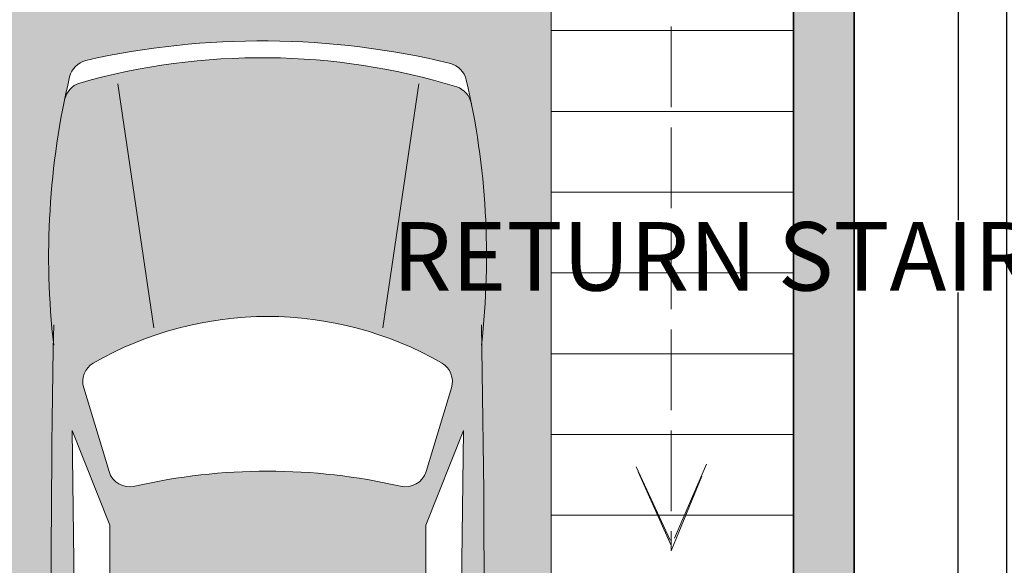
# Model space of a CAD drawing. Units: inches. Extents: x 1077 to 2505, y 1892 to 2728.
# Tile 8 of 26: x 1433 to 1579, y 2176 to 2257. Entities that reach past the tile are written whole.
import ezdxf

# ---------------------------------------------------------------- set-up
doc = ezdxf.new("R2010")
doc.units = ezdxf.units.IN
doc.linetypes.add('ACAD_ISO02W100', pattern=[15, 12, -3])
doc.layers.get('Defpoints').update_dxf_attribs({"color": 220, "linetype": 'ACAD_ISO02W100'})
for name, color, linetype, lineweight in [('A-ANNO-DIMS', 2, 'Continuous', 18), ('A-ANNO-STRS', 220, 'ACAD_ISO02W100', 13), ('A-FLOR-FIXT', 8, 'Continuous', 13), ('A-FLOR-STRS', 7, 'Continuous', 18), ('A-FURNITURE', 251, 'Continuous', 5), ('A-SITE-VEHI', 8, 'Continuous', 13), ('A-WALL-PATT', 7, 'Continuous', 9), ('A_TEXT_SMALL', 18, 'Continuous', 13), ('WALL', 7, 'Continuous', 35)]:
    doc.layers.add(name, color=color, linetype=linetype, lineweight=lineweight)
doc.layers.add('A-FLOR-PATT', color=254, linetype='Continuous', lineweight=9, true_color=0xd7ebd2)
doc.styles.get("Standard").update_dxf_attribs({"font": 'arial.ttf'})
doc.dimstyles.get("Standard").update_dxf_attribs({"dimtxt": 10.18, "dimasz": 0.18, "dimexe": 0.18, "dimexo": 0.0625, "dimgap": 0.09, "dimtad": 0, "dimtih": 1, "dimtoh": 1, "dimdec": 0, "dimzin": 0, "dimdsep": 46, "dimlunit": 3, "dimtxsty": 'Standard', "dimcen": 0.09, "dimadec": 0, "dimazin": 0, "dimtfac": 1, "dimtdec": 0, "dimtofl": 0, "dimtmove": 0, "dimatfit": 3, "dimfxl": 1, "dimtolj": 1, "dimtzin": 0, "dimarcsym": 0})

# ---------------------------------------------------------------- blocks, each defined once
blk = doc.blocks.new('CAR')
at = {"layer": 'A-FURNITURE'}
for p, q in [((2677.91, 1665.57), (2683.24, 1629.33)), ((2722.63, 1665.57), (2717.3, 1629.33)), ((2672.85, 1620.44), (2676.61, 1608)), ((2727.48, 1620.44), (2723.73, 1608)), ((2671.15, 1614.07), (2676.73, 1600.01)), ((2671.63, 1575.61), (2671.15, 1614.07)), ((2729.25, 1614.07), (2723.67, 1600.01)), ((2728.77, 1575.61), (2729.25, 1614.07)), ((2676.73, 1600.01), (2676.73, 1578.97)), ((2723.67, 1600.01), (2723.67, 1578.97)), ((2676.73, 1578.97), (2671.63, 1575.61)), ((2723.67, 1578.97), (2728.77, 1575.61)), ((2676.73, 1576.71), (2671.66, 1573.38)), ((2676.73, 1576.71), (2676.73, 1555.46)), ((2723.67, 1576.71), (2723.67, 1555.46)), ((2723.67, 1576.71), (2728.74, 1573.38)), ((2671.9, 1540.91), (2671.66, 1573.38)), ((2728.49, 1540.91), (2728.74, 1573.38)), ((2676.73, 1555.46), (2671.9, 1540.91)), ((2723.67, 1555.46), (2728.49, 1540.91)), ((2678.77, 1552.01), (2672.52, 1524.85)), ((2721.71, 1552.02), (2727.96, 1524.85)), ((2675.22, 1526.01), (2679.74, 1548.74)), ((2725.17, 1526.01), (2720.66, 1548.74)), ((2672.52, 1524.85), (2672.52, 1517.39)), ((2727.96, 1524.85), (2727.96, 1517.39))]:
    blk.add_line(p, q, dxfattribs=at)
for centre, radius, start, end in [((2699.3, 1552.83), 119.14, 76.3976, 102.667), ((2699.3, 1570.19), 99.28, 73.0347, 105.8141), ((2674, 1665.84), 3.34, 104.3452, 166.6607), ((2726.43, 1665.41), 3.34, 13.1156, 74.5941), ((2783.1, 1639.97), 115.47, 166.6607, 186.5655), ((2673.27, 1662.52), 3.34, 107.8179, 168.3942), ((2727.17, 1661.99), 3.34, 11.3249, 70.8826), ((2617.23, 1639.97), 115.47, 353.4345, 13.1156), ((2700.17, 1579.09), 51.94, 60.0774, 119.9226), ((4741.11, 1589.62), 2073.11, 178.89024, 182.01225), ((659.22, 1589.62), 2073.11, 357.98775, 1.10976), ((2675.91, 1621.37), 3.2, 121.1455, 196.7984), ((2724.42, 1621.37), 3.2, 343.2016, 58.8545), ((2679.67, 1608.92), 3.2, 196.7984, 283.6631), ((2700.17, 1519.83), 88.22, 77.0683, 102.9317), ((2720.66, 1608.92), 3.2, 256.3369, 343.2016), ((2700.16, 1829.45), 278.26, 265.5919, 274.4407), ((2700.17, 1827.63), 279.65, 265.7971, 274.2029), ((2700.17, 1663.47), 139.72, 259.6897, 280.3103), ((2674.03, 1521.04), 4.9, 184.3987, 237.5288), ((2726.3, 1521.04), 4.9, 302.4712, 355.6013), ((2672.62, 1516.95), 3.34, 182.1119, 263.4899), ((2700.17, 1791.26), 275.86, 264.0142, 275.9858), ((2727.71, 1516.95), 3.34, 276.5101, 357.8881), ((2700.17, 1790.18), 277.96, 264.2342, 275.7658)]:
    blk.add_arc(centre, radius, start, end, dxfattribs=at)
blk = doc.blocks.new('reh-flat-2')
at = {"layer": 'A_TEXT_SMALL'}
for p, q in [((486053827.2, -394630231.2), (486054182.4, -394629799.8)), ((486054182.4, -394629799.8), (486054596.6, -394630140.9)), ((486053979.5, -394630126.3), (486054157.1, -394629910.6)), ((486054228.6, -394629903.6), (486054483.5, -394630113.5)), ((486054596.6, -394630140.9), (486054241.4, -394630572.3)), ((486054241.3, -394630407.7), (486053986.4, -394630197.8)), ((486054490.4, -394630185), (486054312.8, -394630400.7)), ((486054241.4, -394630572.3), (486053827.2, -394630231.2))]:
    blk.add_line(p, q, dxfattribs=at)
for centre, radius in [((486054234.9, -394630155.7), 38.1), ((486054004.1, -394630296.2), 20.1), ((486054072.7, -394630352.7), 20.1), ((486054141.4, -394630409.3), 20.1)]:
    blk.add_circle(centre, radius, dxfattribs=at)
for centre, start, end in [((486054196.3, -394629942.9), 50.5305, 140.5305), ((486054018.7, -394630158.5), 140.5305, 230.5305), ((486054451.2, -394630152.8), 320.5305, 50.5305), ((486054273.6, -394630368.4), 230.5305, 320.5305)]:
    blk.add_arc(centre, 50.8, start, end, dxfattribs=at)
blk = doc.blocks.new('*D14')
at = {"layer": 'A-ANNO-DIMS', "color": 0, "lineweight": -2, "transparency": 16777216}
for p, q in [((1555.59, 2651.66), (1579.43, 2651.66)), ((1579.25, 2651.48), (1579.25, 2375.3)), ((1579.25, 2088.54), (1579.25, 2364.72)), ((1555.59, 2088.36), (1579.43, 2088.36))]:
    blk.add_line(p, q, dxfattribs=at)
at = {"layer": 'A-ANNO-DIMS', "color": 0, "transparency": 16777216}
for points in [[(1579.22, 2651.48), (1579.28, 2651.48), (1579.25, 2651.66)], [(1579.22, 2088.54), (1579.28, 2088.54), (1579.25, 2088.36)]]:
    blk.add_solid(points, dxfattribs=at)
at = {"layer": 'Defpoints', "color": 0, "transparency": 16777216}
for p in [(1555.53, 2651.66), (1555.53, 2088.36), (1579.25, 2088.36)]:
    blk.add_point(p, dxfattribs=at)
at = {"layer": 'A-ANNO-DIMS', "color": 0, "transparency": 16777216, "insert": (1579.25, 2370.01), "char_height": 10.18, "attachment_point": 5}
blk.add_mtext('\\A1;46\'-11"', dxfattribs=at)
blk = doc.blocks.new('STAIR-PLAN-RETURN')
for p, q in [((36, 163.08), (36, 0)), ((36, 115.08), (72, 115.08)), ((36, 103.08), (72, 103.08)), ((36, 91.08), (72, 91.08)), ((36, 79.08), (72, 79.08)), ((36, 67.08), (72, 67.08)), ((36, 55.08), (72, 55.08)), ((36, 43.08), (72, 43.08))]:
    blk.add_line(p, q)
blk = doc.blocks.new('STAIR-DIRECTION')
for p, q in [((0, 107.9), (70.51, 107.9)), ((70.51, 107.9), (70.51, 0)), ((70.51, 0.8), (65.28, 12.48)), ((65.28, 12.48), (70.51, 1.21)), ((70.51, 0), (75.75, 12.88)), ((75.75, 12.88), (70.51, 0.8))]:
    blk.add_line(p, q)
blk = doc.blocks.new('*D44')
at = {"layer": 'A-ANNO-DIMS', "color": 0, "lineweight": -2, "transparency": 16777216}
for p, q in [((1547.59, 2303.16), (1572.17, 2303.16)), ((1571.99, 2302.98), (1571.99, 2226.98)), ((1571.99, 2140.26), (1571.99, 2216.26)), ((1547.59, 2140.08), (1572.17, 2140.08))]:
    blk.add_line(p, q, dxfattribs=at)
at = {"layer": 'A-ANNO-DIMS', "color": 0, "transparency": 16777216}
for points in [[(1571.96, 2302.98), (1572.02, 2302.98), (1571.99, 2303.16)], [(1571.96, 2140.26), (1572.02, 2140.26), (1571.99, 2140.08)]]:
    blk.add_solid(points, dxfattribs=at)
at = {"layer": 'Defpoints', "color": 0, "transparency": 16777216}
for p in [(1547.53, 2303.16), (1571.99, 2303.16), (1547.53, 2140.08)]:
    blk.add_point(p, dxfattribs=at)
at = {"layer": 'A-ANNO-DIMS', "color": 0, "transparency": 16777216, "insert": (1571.99, 2221.62), "char_height": 10.18, "attachment_point": 5}
blk.add_mtext('\\A1;RETURN STAIR 13\'-7" TYP.', dxfattribs=at)

msp = doc.modelspace()

# ---------------------------------------------------------------- hatches: boundary and pattern name
at = {"layer": 'A-FLOR-PATT', "transparency": 33554559}
h = msp.add_hatch(color=256, dxfattribs=at)
h.dxf.hatch_style = 1
h.paths.add_polyline_path([(1395.53, 2577.16), (1374.83, 2577.16), (1350.83, 2577.19), (1350.83, 2577.16), (1329.53, 2577.16), (1329.53, 2480.16), (1329.53, 2469.16), (1325.53, 2469.16), (1325.53, 2515.13), (1307.53, 2515.13), (1307.53, 2577.16), (1269.31, 2577.16), (1221.31, 2577.15), (1221.31, 2577.16), (1187.53, 2577.16), (1187.53, 2433.16), (1289.53, 2433.16), (1289.53, 2429.16), (1263.53, 2429.16), (1187.53, 2429.16), (1187.53, 2395.02), (1187.53, 2395.02), (1187.53, 2371.02), (1187.53, 2371.02), (1187.53, 2307.16), (1259.53, 2307.16), (1259.53, 2399.16), (1263.53, 2399.16), (1263.53, 2307.16), (1289.53, 2307.16), (1289.53, 2306.23), (1325.53, 2306.23), (1325.53, 2307.16), (1329.53, 2307.16), (1329.53, 2306.23), (1365.53, 2306.23), (1365.53, 2307.16), (1432.53, 2307.16), (1432.53, 2088.16), (1547.53, 2088.16), (1547.53, 2140.08), (1511.53, 2140.08), (1511.53, 2267.16), (1475.53, 2267.16), (1475.53, 2303.16), (1468.53, 2303.16), (1468.53, 2307.16), (1547.53, 2307.16), (1547.53, 2348.22), (1547.53, 2396.22), (1547.53, 2429.16), (1435.53, 2429.16), (1435.53, 2433.16), (1476.35, 2433.16), (1476.35, 2451.18), (1547.53, 2451.18), (1547.53, 2577.16), (1499.53, 2577.16), (1499.53, 2586.16), (1547.53, 2586.16), (1547.53, 2642.16), (1518.18, 2642.16), (1518.18, 2642.05), (1494.15, 2642.05), (1494.15, 2642.16), (1469.53, 2642.16), (1469.53, 2577.16), (1399.53, 2577.16), (1399.53, 2429.16), (1325.53, 2429.16), (1325.53, 2433.16), (1329.53, 2433.16), (1395.53, 2433.16), (1395.53, 2480.16), (1359.53, 2480.16), (1359.53, 2484.16), (1395.53, 2484.16)])
h.paths.add_polyline_path([(1357.65, 2482.07), (1355.65, 2482.07), (1355.65, 2481.07, 0.414214), (1356.65, 2480.07), (1344.65, 2480.07), (1344.65, 2477.06), (1343.27, 2477.06), (1343.27, 2480.07), (1330.65, 2480.07, -0.414214), (1329.65, 2481.07), (1329.65, 2484.07), (1331.65, 2484.07), (1331.65, 2510.07, -0.446908)], flags=16)
h.paths.add_polyline_path([(1305.09, 2559.18), (1288.89, 2559.18), (1288.89, 2575.38), (1305.09, 2575.38)], flags=16)
h.paths.add_polyline_path([(1304.19, 2560.08), (1289.79, 2560.08), (1289.79, 2574.48), (1304.19, 2574.48)], flags=0)
h.paths.add_polyline_path([(1287.99, 2500.68, -0.414214), (1287.09, 2499.78), (1265.14, 2499.78), (1224.09, 2499.78, -0.414214), (1223.19, 2500.68), (1223.19, 2557.16), (1223.19, 2571.74), (1223.19, 2575.38), (1287.99, 2575.38), (1287.99, 2571.74), (1287.09, 2571.74, -0.414214), (1287.99, 2570.84)], flags=16)
h.paths.add_polyline_path([(1292.98, 2569.05, -1), (1300.92, 2569.05, -1)], flags=0)
h.paths.add_polyline_path([(1293.32, 2569.05, -1), (1300.58, 2569.05, -1)], flags=0)
h.paths.add_polyline_path([(1322.8, 2462.21), (1322.8, 2431.71), (1323.05, 2430.71), (1323.05, 2431.71), (1321.8, 2431.71), (1321.8, 2462.19, 0.404641), (1292.3, 2431.71), (1292.05, 2430.71, -0.414214), (1291.55, 2430.21), (1291.05, 2430.21), (1291.05, 2429.71, -0.414214), (1290.55, 2429.21), (1289.55, 2429.21), (1289.55, 2434.21), (1290.55, 2434.21, -0.414214), (1291.05, 2433.71), (1291.05, 2433.21), (1291.55, 2433.21, -0.414214), (1292.05, 2432.71), (1292.3, 2431.71, -0.414214)], flags=16)
h.paths.add_polyline_path([(1287.82, 2548.28, 0.292232), (1279.17, 2536.8, 0.052719), (1223.93, 2548.28), (1223.28, 2548.28), (1223.28, 2557.16), (1223.93, 2557.16), (1245.42, 2557.16, -0.117785), (1245.77, 2557.93, -0.059418), (1254.87, 2567.02, -0.379859), (1257.28, 2566.88, -0.02509), (1261.41, 2563.32, -0.025935), (1265.65, 2567.02, -0.379859), (1268.06, 2566.88, -0.061767), (1277.52, 2557.43, -0.069393), (1277.82, 2557.16), (1287.82, 2557.16)], flags=0)
h.paths.add_polyline_path([(1263.47, 2548.28), (1260.56, 2548.28, -0.015371), (1258.01, 2546.13, -0.429576), (1255.37, 2546.06, -0.016036), (1252.69, 2548.28), (1223.28, 2548.28), (1223.28, 2554.42), (1246.78, 2554.42, 0.055344), (1255.37, 2546.06, 0.331768), (1257.52, 2545.74, 0.027343), (1262, 2549.64, 0.00919)], flags=0)
h.paths.add_polyline_path([(1295.56, 2568.34), (1296.87, 2569.09), (1296.87, 2570.6, 0.399698), (1295.39, 2569.05, 0.119004)], flags=0)
h.paths.add_polyline_path([(1295.21, 2569.05, -1), (1298.68, 2569.05, -1)], flags=0)
h.paths.add_polyline_path([(1296.95, 2568.96), (1297.03, 2569), (1297.03, 2569.09), (1296.99, 2569.11), (1296.91, 2568.98)], flags=0)
h.paths.add_polyline_path([(1402.28, 2462.19, -0.414214), (1432.78, 2431.69), (1433.03, 2432.69), (1432.78, 2431.69, 0.404641), (1403.28, 2462.17), (1403.28, 2431.69), (1402.03, 2431.69), (1402.03, 2430.69, -0.414214), (1401.53, 2430.19), (1401.03, 2430.19), (1401.03, 2429.69, -0.414214), (1400.53, 2429.19), (1399.53, 2429.19), (1399.53, 2434.19), (1400.53, 2434.19, -0.414214), (1401.03, 2433.69), (1401.03, 2433.19), (1401.53, 2433.19, -0.414214), (1402.03, 2432.69)], flags=16)
h.paths.add_polyline_path([(1470.16, 2535.21, -0.414214), (1471.06, 2536.11), (1527.54, 2536.11), (1542.12, 2536.11), (1545.76, 2536.11), (1545.76, 2471.31), (1542.12, 2471.31), (1542.12, 2472.21, -0.414214), (1541.22, 2471.31), (1471.06, 2471.31, -0.414214), (1470.16, 2472.21), (1470.16, 2494.16)], flags=16)
h.paths.add_polyline_path([(1483.07, 2536.11, 0.253465), (1480.11, 2526.15, 0.2538), (1470.15, 2523.19)], flags=16)
h.paths.add_polyline_path([(1223.19, 2512.69, 0.253465), (1233.14, 2509.74, 0.2538), (1236.1, 2499.77)], flags=16)
h.paths.add_polyline_path([(1469.77, 2578.72), (1469.77, 2581.72), (1471.77, 2581.72), (1471.77, 2607.72, -0.01951), (1473.77, 2607.68), (1473.77, 2579.72), (1473.77, 2578.72, -0.414214), (1472.77, 2577.72), (1470.77, 2577.72, -0.414214)], flags=16)
h.paths.add_polyline_path([(1382.46, 2398.13), (1395.04, 2398.13), (1395.04, 2399.74), (1382.46, 2399.74)], flags=16)
h.paths.add_polyline_path([(1379.94, 2397.18), (1379.94, 2389.82), (1380.5, 2389.82), (1380.5, 2396.05, -0.41429), (1381.06, 2396.61), (1396.47, 2396.61, -0.414213), (1397.03, 2396.05), (1397.03, 2389.82), (1397.59, 2389.82), (1397.59, 2397.18)], flags=16)
h.paths.add_polyline_path([(1263.37, 2428.14), (1263.37, 2426.14, -0.414214), (1262.37, 2425.14), (1261.37, 2425.14), (1233.41, 2425.14, 0.400854), (1259.37, 2401.04), (1259.37, 2401.14), (1261.37, 2401.14, -0.446908), (1233.37, 2427.14), (1259.37, 2427.14), (1259.37, 2429.14), (1262.37, 2429.14, -0.414214)], flags=16)
h.paths.add_polyline_path([(1404.79, 2398.13), (1417.37, 2398.13), (1417.37, 2399.74), (1404.79, 2399.74)], flags=16)
h.paths.add_polyline_path([(1402.27, 2397.18), (1404.79, 2398.13), (1417.37, 2398.13), (1419.92, 2397.18)], flags=16)
h.paths.add_polyline_path([(1432.26, 2383.16), (1432.26, 2370.59), (1433.87, 2370.59), (1433.87, 2383.16)], flags=16)
h.paths.add_polyline_path([(1431.3, 2385.69), (1423.84, 2385.69), (1423.84, 2385.13), (1430.18, 2385.13, -0.41429), (1430.74, 2384.57), (1430.74, 2369.16, -0.414237), (1430.18, 2368.6), (1423.84, 2368.6), (1423.84, 2368.03), (1431.3, 2368.03)], flags=16)
h.paths.add_polyline_path([(1417.37, 2351.16), (1417.37, 2349.54), (1418.9, 2349.54, 0.414236), (1419.92, 2350.56), (1419.92, 2352.11)], flags=16)
h.paths.add_polyline_path([(1395.04, 2351.16), (1395.04, 2349.54), (1396.58, 2349.54, 0.414235), (1397.59, 2350.56), (1397.59, 2352.11)], flags=16)
h.paths.add_polyline_path([(1366.7, 2370.05), (1365.09, 2370.05), (1365.09, 2368.52, 0.414235), (1366.11, 2367.5), (1367.66, 2367.5)], flags=16)
h.paths.add_polyline_path([(1419.36, 2359.47), (1419.36, 2353.24, -0.41419), (1418.8, 2352.68), (1403.39, 2352.68, -0.414137), (1402.83, 2353.24), (1402.83, 2359.47), (1397.03, 2359.47), (1397.03, 2353.24, -0.414189), (1396.47, 2352.68), (1381.06, 2352.68, -0.414137), (1380.5, 2353.24), (1380.5, 2359.47)], flags=16)
h.paths.add_polyline_path([(1222.29, 2559.18), (1206.09, 2559.18), (1206.09, 2575.38), (1222.29, 2575.38)], flags=16)
h.paths.add_polyline_path([(1221.39, 2560.08), (1206.99, 2560.08), (1206.99, 2574.48), (1221.39, 2574.48)], flags=0)
h.paths.add_polyline_path([(1482, 2577.72), (1482, 2580.73), (1483.38, 2580.73), (1483.38, 2577.72), (1484.77, 2577.72), (1484.77, 2574.72), (1483.38, 2574.72), (1483.38, 2577.72)], flags=16)
h.paths.add_polyline_path([(1266.37, 2415.53), (1266.37, 2414.14), (1263.37, 2414.14), (1263.37, 2415.53), (1260.36, 2415.53), (1260.36, 2416.91), (1263.37, 2416.91), (1263.37, 2415.53)], flags=16)
h.paths.add_polyline_path([(1210.26, 2569.05, -1), (1218.19, 2569.05, -1)], flags=0)
h.paths.add_polyline_path([(1210.6, 2569.05, -1), (1217.85, 2569.05, -1)], flags=0)
h.paths.add_polyline_path([(1212.84, 2568.34), (1214.15, 2569.09), (1214.15, 2570.6, 0.399698), (1212.67, 2569.05, 0.119004)], flags=0)
h.paths.add_polyline_path([(1212.49, 2569.05, -1), (1215.96, 2569.05, -1)], flags=0)
h.paths.add_polyline_path([(1214.23, 2568.96), (1214.3, 2568.91), (1214.3, 2569)], flags=0)
h.paths.add_polyline_path([(1507.18, 2480.12, 0.052719), (1518.66, 2535.36), (1518.66, 2536.01), (1527.54, 2536.01), (1527.54, 2535.36), (1527.54, 2513.88, -0.117785), (1528.31, 2513.53, -0.059418), (1537.4, 2504.43, -0.379859), (1537.26, 2502.01, -0.02509), (1533.7, 2497.89, -0.025935), (1537.4, 2493.64, -0.379859), (1537.26, 2491.23, -0.061767), (1527.8, 2481.77, -0.069393), (1527.54, 2481.47), (1527.54, 2471.47), (1518.66, 2471.47, 0.292232)], flags=0)
h.paths.add_polyline_path([(1516.43, 2503.92, -0.016036), (1518.66, 2506.6), (1518.66, 2536.01), (1524.8, 2536.01), (1524.8, 2512.51, 0.055344), (1516.43, 2503.92, 0.331768), (1516.12, 2501.77, 0.027343), (1520.01, 2497.29, 0.00919), (1518.66, 2495.82), (1518.66, 2498.73, -0.015371), (1516.5, 2501.28, -0.429576)], flags=0)
h.paths.add_polyline_path([(1499.63, 2625.5, -0.171636), (1502.82, 2631.01), (1502.82, 2633.37), (1498.68, 2633.37, -0.414214), (1497.7, 2634.36), (1497.7, 2640.66, -0.414214), (1498.68, 2641.64), (1514.82, 2641.64, -0.414214), (1515.81, 2640.66), (1515.81, 2634.36, -0.414214), (1514.82, 2633.37), (1510.69, 2633.37), (1510.69, 2631.01, -0.171636), (1513.88, 2625.5, -0.258205), (1509.31, 2614.47), (1504.19, 2614.47, -0.258205)], flags=16)
h.paths.add_polyline_path([(1501.2, 2625.5, -0.171636), (1504.39, 2631.01), (1509.12, 2631.01, -0.171636), (1512.3, 2625.5, -0.210384), (1509.35, 2616.02), (1504.16, 2616.02, -0.210384)], flags=0)
h.paths.add_polyline_path([(1529.56, 2537.01), (1529.56, 2553.21), (1545.76, 2553.21), (1545.76, 2537.01)], flags=16)
h.paths.add_polyline_path([(1530.46, 2537.91), (1530.46, 2552.31), (1544.86, 2552.31), (1544.86, 2537.91)], flags=0)
h.paths.add_polyline_path([(1535.45, 2545.07, -1), (1543.39, 2545.07, -1)], flags=0)
h.paths.add_polyline_path([(1535.8, 2545.07, -1), (1543.05, 2545.07, -1)], flags=0)
h.paths.add_polyline_path([(1529.56, 2470.41), (1545.76, 2470.41), (1545.76, 2454.21), (1529.56, 2454.21)], flags=16)
h.paths.add_polyline_path([(1541.16, 2544.99), (1540.98, 2544.99, -0.544606), (1538.71, 2543.68), (1538.62, 2543.53, 0.547962)], flags=0)
h.paths.add_polyline_path([(1530.46, 2469.51), (1544.86, 2469.51), (1544.86, 2455.11), (1530.46, 2455.11)], flags=0)
h.paths.add_polyline_path([(1539.47, 2545.14), (1539.42, 2545.22), (1539.38, 2545.14)], flags=0)
h.paths.add_polyline_path([(1543.39, 2462.34, -1), (1535.45, 2462.34, -1)], flags=0)
h.paths.add_polyline_path([(1543.05, 2462.34, -1), (1535.8, 2462.34, -1)], flags=0)
h.paths.add_polyline_path([(1541.16, 2462.27), (1540.98, 2462.27, -0.544606), (1538.71, 2460.96), (1538.62, 2460.8, 0.547962)], flags=0)
h.paths.add_polyline_path([(1539.47, 2462.42), (1539.42, 2462.5), (1539.38, 2462.42)], flags=0)
h.paths.add_polyline_path([(1435.32, 2335.25, -0.414214), (1465.82, 2304.75), (1466.07, 2305.75), (1465.82, 2304.75, 0.404641), (1436.32, 2335.23), (1436.32, 2304.75), (1435.07, 2304.75), (1435.07, 2303.75, -0.414214), (1434.57, 2303.25), (1434.07, 2303.25), (1434.07, 2302.75, -0.414214), (1433.57, 2302.25), (1432.57, 2302.25), (1432.57, 2307.25), (1433.57, 2307.25, -0.414214), (1434.07, 2306.75), (1434.07, 2306.25), (1434.57, 2306.25, -0.414214), (1435.07, 2305.75)], flags=16)
h.paths.add_polyline_path([(1532.13, 2635.71), (1535.43, 2635.71), (1535.43, 2635.89), (1532.13, 2635.89)], flags=16)
edge = h.paths.add_edge_path(flags=16)
edge.add_arc((1535.98, 2632.67), 0.183, 270, 360)
edge.add_line((1536.17, 2632.67), (1536.17, 2639.82))
edge.add_line((1536.17, 2639.82), (1538.29, 2639.82))
edge.add_line((1538.29, 2639.82), (1538.29, 2641.82))
edge.add_line((1538.29, 2641.82), (1533.25, 2641.82))
edge.add_line((1533.25, 2641.82), (1533.25, 2639.82))
edge.add_line((1533.25, 2639.82), (1534.87, 2639.82))
edge.add_line((1534.87, 2639.82), (1534.87, 2639))
edge.add_line((1534.87, 2639), (1533.7, 2639))
edge.add_line((1533.7, 2639), (1533.7, 2639.82))
edge.add_line((1533.7, 2639.82), (1533.25, 2639.82))
edge.add_line((1533.25, 2639.82), (1533.25, 2641.82))
edge.add_line((1533.25, 2641.82), (1538.29, 2641.82))
edge.add_line((1538.29, 2641.82), (1538.29, 2641.34))
edge.add_line((1538.29, 2641.34), (1540.64, 2641.58))
edge.add_line((1540.64, 2641.58), (1540.64, 2641.82))
edge.add_line((1540.64, 2641.82), (1541.5, 2641.82))
edge.add_line((1541.5, 2641.82), (1541.5, 2641.25))
edge.add_line((1541.5, 2641.25), (1541.31, 2639.79))
edge.add_ellipse((1541.09, 2638.95), major_axis=(-1.08, 0), ratio=0.790849, start_angle=180, end_angle=255.2976, ccw=False)
edge.add_line((1542.17, 2638.95), (1542.17, 2638.38))
edge.add_ellipse((1541.09, 2638.38), major_axis=(-1.08, 0), ratio=0.790849, start_angle=0, end_angle=180, ccw=False)
edge.add_line((1540, 2638.38), (1540.01, 2638.87))
edge.add_ellipse((1541.09, 2638.95), major_axis=(-1.08, 0), ratio=0.790849, start_angle=284.7024, end_angle=364.0401, ccw=False)
edge.add_line((1540.78, 2639.75), (1540.78, 2641.25))
edge.add_line((1540.78, 2641.25), (1540.64, 2641.25))
edge.add_line((1540.64, 2641.25), (1538.29, 2641.01))
edge.add_line((1538.29, 2641.01), (1538.29, 2639.82))
edge.add_line((1538.29, 2639.82), (1536.17, 2639.82))
edge.add_line((1536.17, 2639.82), (1536.17, 2632.48))
edge.add_line((1536.17, 2632.48), (1535.98, 2632.48))
h.paths.add_polyline_path([(1496.32, 2250.34, -0.292371), (1498.9, 2247.83, -0.085148), (1501.21, 2208.85, -0.01331), (1500.27, 2098.5, -0.379287), (1497.22, 2095.28, -0.0502), (1441.54, 2095.28, -0.379287), (1438.5, 2098.5, -0.01331), (1437.56, 2208.85, -0.086132), (1439.96, 2248.26, -0.295116), (1442.59, 2250.78, -0.114238)], flags=16)
h.paths.add_polyline_path([(1495.16, 2205.84, -0.355389), (1496.7, 2202.1), (1492.94, 2189.65, -0.398275), (1489.12, 2187.47, 0.113332), (1449.64, 2187.47, -0.398275), (1445.82, 2189.65), (1442.06, 2202.1, -0.355394), (1443.6, 2205.84, -0.265725)], flags=0)
h.paths.add_polyline_path([(1440.37, 2195.72), (1445.94, 2181.67), (1445.94, 2160.63), (1440.84, 2157.26)], flags=0)
h.paths.add_polyline_path([(1498.46, 2195.72), (1497.99, 2157.26), (1492.88, 2160.63), (1492.88, 2181.67)], flags=0)
h.paths.add_polyline_path([(1445.94, 2158.37), (1445.94, 2137.12), (1441.12, 2122.56), (1440.87, 2155.03)], flags=0)
h.paths.add_polyline_path([(1492.88, 2158.37), (1497.96, 2155.03), (1497.71, 2122.56), (1492.88, 2137.12)], flags=0)
h.paths.add_polyline_path([(1489.88, 2130.4), (1494.39, 2107.67, -0.090102), (1444.44, 2107.65), (1448.95, 2130.39, 0.036636)], flags=0)
h.paths.add_polyline_path([(1447.54, 2159.34), (1497.44, 2159.34), (1497.44, 2177.89), (1447.54, 2177.89)], flags=8)
h.paths.add_polyline_path([(1196.44, 2354.84), (1246.65, 2354.84), (1246.65, 2388.43), (1196.44, 2388.43)], flags=24)
h.paths.add_polyline_path([(1296.09, 2360.25), (1353.81, 2360.25), (1353.81, 2393.84), (1296.09, 2393.84)], flags=24)
h.paths.add_polyline_path([(1400.72, 2471.85), (1470.63, 2471.85), (1470.63, 2505.44), (1400.72, 2505.44)], flags=24)
h.paths.add_polyline_path([(1324.78, 2448.48), (1394.95, 2448.48), (1394.95, 2467.02), (1324.78, 2467.02)], flags=24)
h.paths.add_polyline_path([(1335.08, 2531.43), (1389.67, 2531.43), (1389.67, 2565.02), (1335.08, 2565.02)], flags=24)
h.paths.add_polyline_path([(1225.76, 2460), (1295.67, 2460), (1295.67, 2493.58), (1225.76, 2493.58)], flags=24)
h = msp.add_hatch(color=256, dxfattribs=at)
h.dxf.hatch_style = 1
h.paths.add_polyline_path([(1547.53, 2348.22), (1547.53, 2396.22), (1547.53, 2425.11), (1547.53, 2425.11), (1547.53, 2429.16), (1435.53, 2429.16), (1434.03, 2429.21), (1434.03, 2430.19), (1433.03, 2430.19), (1432.78, 2431.69, 0.404641), (1403.28, 2462.17), (1403.28, 2431.69), (1402.03, 2431.69), (1402.03, 2430.19), (1401.03, 2430.19), (1401.03, 2429.19), (1399.53, 2429.19), (1399.53, 2429.19), (1399.53, 2429.16), (1334.67, 2429.16), (1334.67, 2423.95), (1325.67, 2423.95), (1325.67, 2429.16), (1325.53, 2429.16), (1324.05, 2429.24), (1324.05, 2430.21), (1323.05, 2430.21), (1323.05, 2431.71), (1321.8, 2431.71), (1321.8, 2462.19, 0.416544), (1292.05, 2430.73, -0.423614), (1291.55, 2430.21), (1291.05, 2430.21), (1291.05, 2429.21), (1289.55, 2429.21), (1289.53, 2429.21), (1289.53, 2429.16), (1263.37, 2429.16), (1263.37, 2415.53), (1266.37, 2415.53), (1266.37, 2414.14), (1263.37, 2414.14), (1263.37, 2399.16), (1263.53, 2399.16), (1263.53, 2307.16), (1289.53, 2307.16), (1289.53, 2306.23), (1323.26, 2306.23), (1323.26, 2307.21), (1332.26, 2307.21), (1365.53, 2306.23), (1365.53, 2307.16), (1432.53, 2307.16), (1432.57, 2307.16), (1432.57, 2307.25), (1434.07, 2307.25), (1434.07, 2306.25), (1435.32, 2306.25), (1435.32, 2335.25, -0.407346), (1466.07, 2305.73, -0.423614), (1466.57, 2306.25), (1467.07, 2306.25), (1467.07, 2307.25), (1468.57, 2307.25), (1547.53, 2307.16), (1547.53, 2307.2)])
h.paths.add_polyline_path([(1430.74, 2369.16), (1430.74, 2384.57, 0.41429), (1430.18, 2385.13), (1423.84, 2385.13), (1423.84, 2368.6), (1430.18, 2368.6, 0.414237)], flags=16)
h.paths.add_polyline_path([(1432.26, 2383.16), (1432.26, 2370.59), (1433.87, 2370.59), (1433.87, 2383.16)], flags=16)
h.paths.add_polyline_path([(1431.3, 2368.03), (1431.3, 2385.69), (1432.26, 2383.16), (1432.26, 2370.59)], flags=16)
h.paths.add_polyline_path([(1417.37, 2351.16), (1417.37, 2349.54), (1418.9, 2349.54, 0.414236), (1419.92, 2350.56), (1419.92, 2352.11)], flags=16)
h.paths.add_polyline_path([(1403.39, 2352.68), (1418.78, 2352.68, 0.42427), (1419.36, 2353.24), (1419.36, 2359.47), (1402.83, 2359.47), (1402.83, 2353.24, 0.414137)], flags=16)
h.paths.add_polyline_path([(1366.7, 2370.05), (1365.09, 2370.05), (1365.09, 2368.52, 0.414235), (1366.11, 2367.5), (1367.66, 2367.5)], flags=16)
h.paths.add_polyline_path([(1382.46, 2398.13), (1395.04, 2398.13), (1395.04, 2399.74), (1382.46, 2399.74)], flags=16)
h.paths.add_polyline_path([(1396.47, 2396.61), (1381.06, 2396.61, 0.41429), (1380.5, 2396.05), (1380.5, 2389.82), (1397.03, 2389.82), (1397.03, 2396.05, 0.414213)], flags=16)
h.paths.add_polyline_path([(1402.27, 2397.18), (1402.83, 2396.05, -0.414213), (1403.39, 2396.61)], flags=16)
h.paths.add_polyline_path([(1418.8, 2396.61), (1419.36, 2396.61), (1419.36, 2396.05, 0.414237)], flags=16)
h.paths.add_polyline_path([(1404.79, 2398.13), (1417.37, 2398.13), (1417.37, 2399.74), (1404.79, 2399.74)], flags=16)
h.paths.add_polyline_path([(1381.06, 2352.68, -0.414213), (1380.5, 2353.24), (1380.27, 2352.11)], flags=16)
h.paths.add_polyline_path([(1396.58, 2349.54), (1396.58, 2349.54), (1395.04, 2349.54), (1395.04, 2349.54), (1382.46, 2349.54), (1382.46, 2351.16), (1395.04, 2351.16), (1397.59, 2352.11), (1397.59, 2350.56, -0.414235)], flags=16)
h.paths.add_polyline_path([(1379.94, 2397.18), (1382.46, 2398.13), (1395.04, 2398.13), (1397.59, 2397.18)], flags=16)
h.paths.add_polyline_path([(1368.78, 2384.59, 0.414213), (1368.22, 2384.03), (1367.66, 2367.5), (1367.66, 2385.15)], flags=16)
h.paths.add_polyline_path([(1547.53, 2574.38), (1547.51, 2574.38), (1547.51, 2577.16), (1499.53, 2577.16), (1484.77, 2577.44), (1484.77, 2574.72), (1483.38, 2574.72), (1483.38, 2577.72), (1482, 2577.72), (1469.53, 2577.72), (1469.53, 2577.16), (1401.95, 2577.16), (1401.95, 2574.12), (1399.53, 2574.12), (1399.53, 2434.19), (1401.03, 2434.19), (1401.03, 2433.19), (1402.28, 2433.19), (1402.28, 2462.19, -0.407346), (1433.03, 2432.67, -0.423614), (1433.53, 2433.19), (1434.03, 2433.19), (1434.03, 2434.19), (1435.53, 2434.19), (1476.35, 2433.81), (1476.35, 2451.18), (1547.53, 2451.18)])
h.paths.add_polyline_path([(1470.16, 2535.21, -0.414214), (1471.06, 2536.11), (1527.54, 2536.11), (1542.12, 2536.11), (1545.76, 2536.11), (1545.76, 2471.31), (1542.12, 2471.31), (1542.12, 2472.21, -0.414214), (1541.22, 2471.31), (1471.06, 2471.31, -0.414214), (1470.16, 2472.21), (1470.16, 2494.16)], flags=16)
h.paths.add_polyline_path([(1483.07, 2536.11, 0.253465), (1480.11, 2526.15, 0.2538), (1470.15, 2523.19)], flags=16)
h.paths.add_polyline_path([(1525.55, 2481.52, -0.000893), (1524.8, 2482.24), (1524.8, 2471.47), (1527.54, 2471.47), (1527.54, 2472.12), (1527.54, 2481.47, -0.388819)], flags=0)
h.paths.add_polyline_path([(1518.66, 2536.01), (1527.54, 2536.01), (1527.54, 2535.36), (1527.54, 2513.88, -0.117785), (1528.31, 2513.53, -0.059418), (1537.4, 2504.43, -0.379859), (1537.26, 2502.01, -0.02509), (1533.7, 2497.89, 0.033431), (1528.3, 2502.74, 0.308459), (1526.25, 2502.88, 0.047827), (1518.66, 2495.82), (1518.66, 2498.73, -0.015371), (1516.5, 2501.28, -0.429576), (1516.43, 2503.92, -0.016036), (1518.66, 2506.6)], flags=0)
h.paths.add_polyline_path([(1529.56, 2537.01), (1529.56, 2553.21), (1545.76, 2553.21), (1545.76, 2537.01)], flags=16)
h.paths.add_polyline_path([(1530.46, 2537.91), (1530.46, 2552.31), (1544.86, 2552.31), (1544.86, 2537.91)], flags=0)
h.paths.add_polyline_path([(1535.8, 2545.07, -1), (1543.05, 2545.07, -1)], flags=0)
h.paths.add_polyline_path([(1541.16, 2544.99), (1540.98, 2544.99, -0.544606), (1538.71, 2543.68), (1538.62, 2543.53, 0.547962)], flags=0)
h.paths.add_polyline_path([(1539.47, 2545.14), (1539.42, 2545.22), (1539.38, 2545.14)], flags=0)
h.paths.add_polyline_path([(1529.56, 2470.41), (1545.76, 2470.41), (1545.76, 2454.21), (1529.56, 2454.21)], flags=16)
h.paths.add_polyline_path([(1530.46, 2469.51), (1544.86, 2469.51), (1544.86, 2455.11), (1530.46, 2455.11)], flags=0)
h.paths.add_polyline_path([(1535.8, 2462.34, -1), (1543.05, 2462.34, -1)], flags=0)
h.paths.add_polyline_path([(1541.16, 2462.27), (1540.98, 2462.27, -0.544606), (1538.71, 2460.96), (1538.62, 2460.8, 0.547962)], flags=0)
h.paths.add_polyline_path([(1539.47, 2462.42), (1539.42, 2462.5), (1539.38, 2462.42)], flags=0)
h.paths.add_polyline_path([(1395.53, 2574.12), (1392.95, 2574.12), (1392.95, 2577.16), (1374.83, 2577.16), (1350.83, 2577.19), (1350.83, 2577.16), (1332.07, 2577.16), (1332.07, 2574), (1329.53, 2574), (1329.53, 2484.07), (1331.65, 2484.07), (1331.65, 2510.07, -0.423677), (1357.76, 2484.07), (1359.53, 2484.07), (1359.53, 2484.16), (1395.53, 2484.16)], flags=17)
h.paths.add_polyline_path([(1395.53, 2480.16), (1359.06, 2480.16, 0.437533), (1359.53, 2481.55), (1359.53, 2484.16), (1395.53, 2484.16), (1395.53, 2574.12), (1392.95, 2574.12), (1392.95, 2577.16), (1374.83, 2577.16), (1350.83, 2577.19), (1350.83, 2577.16), (1332.07, 2577.16), (1332.07, 2574), (1329.53, 2574), (1329.53, 2484.07), (1329.65, 2484.07), (1329.65, 2481.07), (1329.53, 2480.16), (1329.53, 2469.16), (1325.53, 2469.16), (1325.53, 2515.13), (1307.53, 2515.13), (1307.53, 2577.16), (1269.31, 2577.16), (1221.31, 2577.15), (1221.31, 2577.16), (1187.61, 2577.16), (1187.61, 2574.03), (1187.53, 2433.16), (1289.55, 2433.16), (1289.55, 2434.21), (1291.05, 2434.21), (1291.05, 2433.21), (1292.05, 2433.21), (1292.3, 2431.71, -0.414214), (1322.8, 2462.21), (1323.05, 2432.71, -0.414214), (1323.55, 2433.21), (1324.05, 2433.21), (1324.05, 2434.21), (1325.67, 2434.21), (1325.67, 2435.95), (1334.67, 2435.95), (1334.67, 2433.16), (1395.53, 2433.16)])
h.paths.add_polyline_path([(1344.65, 2480.07), (1344.65, 2477.06), (1343.27, 2477.06), (1343.27, 2480.07), (1332.65, 2480.07, 0.414214), (1333.65, 2481.07), (1333.65, 2482.07), (1331.65, 2482.07), (1331.65, 2484.07), (1331.65, 2510.07, -0.446908), (1357.65, 2482.07), (1355.65, 2482.07), (1355.65, 2481.07, 0.414214), (1356.65, 2480.07)], flags=16)
h.paths.add_polyline_path([(1287.99, 2500.68, -0.414214), (1287.09, 2499.78), (1265.14, 2499.78), (1224.09, 2499.78, -0.414214), (1223.19, 2500.68), (1223.19, 2557.16), (1223.19, 2571.74), (1223.19, 2575.38), (1287.99, 2575.38), (1287.99, 2571.74), (1287.09, 2571.74, -0.414214), (1287.99, 2570.84)], flags=16)
h.paths.add_polyline_path([(1277.77, 2555.17, -0.000893), (1277.05, 2554.42), (1287.82, 2554.42), (1287.82, 2557.16), (1287.17, 2557.16), (1277.82, 2557.16, -0.388819)], flags=0)
h.paths.add_polyline_path([(1223.28, 2548.28), (1223.28, 2557.16), (1223.93, 2557.16), (1245.42, 2557.16, -0.117785), (1245.77, 2557.93, -0.059418), (1254.87, 2567.02, -0.379859), (1257.28, 2566.88, -0.02509), (1261.41, 2563.32, 0.033431), (1256.55, 2557.93, 0.308459), (1256.41, 2555.88, 0.047827), (1263.47, 2548.28), (1260.56, 2548.28, -0.015371), (1258.01, 2546.13, -0.429576), (1255.37, 2546.06, -0.016036), (1252.69, 2548.28)], flags=0)
h.paths.add_polyline_path([(1305.09, 2559.18), (1288.89, 2559.18), (1288.89, 2575.38), (1305.09, 2575.38)], flags=16)
h.paths.add_polyline_path([(1304.19, 2560.08), (1289.79, 2560.08), (1289.79, 2574.48), (1304.19, 2574.48)], flags=0)
h.paths.add_polyline_path([(1300.58, 2569.05, -1), (1293.32, 2569.05, -1)], flags=0)
h.paths.add_polyline_path([(1223.19, 2512.69, 0.253465), (1233.14, 2509.74, 0.2538), (1236.1, 2499.77)], flags=16)
h.paths.add_polyline_path([(1295.56, 2568.34), (1296.87, 2569.09), (1296.87, 2570.6, 0.399698), (1295.39, 2569.05, 0.119004)], flags=0)
h.paths.add_polyline_path([(1295.21, 2569.05, -1), (1298.68, 2569.05, -1)], flags=0)
h.paths.add_polyline_path([(1296.95, 2568.96), (1297.03, 2569), (1297.03, 2569.09), (1296.99, 2569.11), (1296.91, 2568.98)], flags=0)
h.paths.add_polyline_path([(1222.29, 2559.18), (1206.09, 2559.18), (1206.09, 2575.38), (1222.29, 2575.38)], flags=16)
h.paths.add_polyline_path([(1221.39, 2560.08), (1206.99, 2560.08), (1206.99, 2574.48), (1221.39, 2574.48)], flags=0)
h.paths.add_polyline_path([(1217.85, 2569.05, -1), (1210.6, 2569.05, -1)], flags=0)
h.paths.add_polyline_path([(1212.84, 2568.34), (1214.15, 2569.09), (1214.15, 2570.6, 0.399698), (1212.67, 2569.05, 0.119004)], flags=0)
h.paths.add_polyline_path([(1212.49, 2569.05, -1), (1215.96, 2569.05, -1)], flags=0)
h.paths.add_polyline_path([(1214.23, 2568.96), (1214.3, 2569), (1214.3, 2569.09), (1214.26, 2569.11), (1214.19, 2568.98)], flags=0)
h.paths.add_polyline_path([(1259.53, 2399.14), (1259.37, 2399.14), (1259.37, 2401.04, -0.423677), (1233.37, 2427.14), (1259.37, 2427.14), (1259.37, 2429.16), (1187.53, 2429.16), (1187.53, 2395.02), (1187.53, 2395.02), (1187.53, 2371.02), (1187.53, 2371.02), (1187.53, 2311.49), (1187.55, 2311.49), (1187.55, 2307.16), (1259.53, 2307.16)])
h.paths.add_polyline_path([(1323.26, 2295.21), (1323.26, 2304.23), (1289.53, 2304.23), (1289.53, 2303.16), (1187.55, 2303.16), (1187.55, 2299.49), (1178.53, 2299.49), (1178.53, 2267.66), (1178.53, 2219.66), (1182.03, 2219.66), (1182.03, 2267.67), (1184.03, 2267.67), (1184.03, 2219.66), (1187.53, 2219.66), (1187.53, 2153.16), (1228.13, 2153.16), (1276.13, 2153.16), (1276.13, 2153.16), (1324.54, 2153.16), (1324.54, 2154.67), (1325.54, 2154.67), (1325.54, 2155.92), (1296.54, 2155.92, -0.407346), (1326.06, 2186.67, -0.423614), (1325.54, 2187.17), (1325.54, 2187.67), (1324.54, 2187.67), (1324.54, 2189.17), (1325.43, 2295.21)])
h.paths.add_polyline_path([(1432.53, 2307.16), (1365.53, 2307.16), (1365.53, 2306.23), (1365.53, 2303.16), (1428.53, 2303.16), (1428.53, 2221.2), (1428.57, 2221.2), (1428.57, 2197.2), (1428.53, 2197.16), (1428.53, 2303.01), (1404.46, 2303.01), (1404.46, 2221.2), (1329.53, 2221.2), (1329.53, 2307.16), (1325.53, 2307.16), (1325.53, 2295.21), (1325.43, 2295.21), (1324.54, 2189.17), (1324.54, 2187.67), (1326.04, 2187.67, 1.016365), (1326.06, 2186.67, 0.407348), (1296.54, 2155.92), (1325.54, 2155.92), (1325.54, 2154.67), (1324.54, 2154.67), (1324.54, 2153.16), (1329.53, 2153.16), (1329.53, 2144.16), (1432.53, 2144.16)])
h.paths.add_polyline_path([(1361.95, 2194.26), (1361.95, 2193.16), (1329.53, 2193.16), (1329.53, 2189.16), (1329.54, 2188.17), (1329.54, 2189.16), (1329.53, 2189.16), (1329.53, 2193.16), (1361.95, 2193.16), (1361.95, 2196.26), (1409.95, 2196.26), (1409.95, 2194.26)], flags=16)
h.paths.add_polyline_path([(1377.02, 2200.5), (1345.91, 2200.5), (1345.91, 2218.4), (1347.87, 2218.4), (1347.87, 2219.18), (1374.75, 2219.18), (1374.75, 2218.4), (1377.02, 2218.4)], flags=16)
h.paths.add_polyline_path([(1367.07, 2210.7, -1), (1373.34, 2210.7, -1)], flags=0)
h.paths.add_polyline_path([(1349.92, 2210.7, -1), (1356.98, 2210.7, -1)], flags=0)
h.paths.add_polyline_path([(1405.95, 2256.57), (1405.95, 2277.6), (1427.86, 2277.6), (1427.86, 2256.57)], flags=16)
h.paths.add_polyline_path([(1412.92, 2258.68, -0.414201), (1410.93, 2260.67), (1410.93, 2273.62, -0.414239), (1412.92, 2275.61), (1423.88, 2275.61, -0.414227), (1425.87, 2273.62), (1425.87, 2260.67, -0.414214), (1423.88, 2258.68)], flags=0)
h.paths.add_polyline_path([(1407.61, 2263.66, -1), (1409.18, 2263.66, -1)], flags=0)
h.paths.add_polyline_path([(1407.61, 2267.14, -1), (1409.18, 2267.14, -1)], flags=0)
h.paths.add_polyline_path([(1416.91, 2267.15, -1), (1419.89, 2267.15, -1)], flags=0)
h.paths.add_polyline_path([(1407.61, 2270.63, -1), (1409.18, 2270.63, -1)], flags=0)
h.paths.add_polyline_path([(1475.53, 2303.16), (1468.57, 2303.16), (1468.57, 2302.25), (1467.07, 2302.25), (1467.07, 2303.25), (1466.07, 2303.25), (1465.82, 2304.75, 0.404641), (1436.32, 2335.23), (1436.32, 2304.75), (1435.07, 2304.75), (1435.07, 2303.25), (1434.07, 2303.25), (1434.07, 2302.25), (1432.53, 2302.25), (1432.53, 2144.16), (1432.53, 2088.16), (1547.52, 2088.16), (1547.52, 2100.19), (1547.52, 2140.08), (1511.53, 2140.08), (1511.53, 2267.16), (1475.53, 2267.16)])
h.paths.add_polyline_path([(1438.35, 2102.86, 0.033498), (1438.37, 2102.21, -0.000079)], flags=16)
h.paths.add_polyline_path([(1496.32, 2250.34, -0.292371), (1498.9, 2247.83, -0.085148), (1501.21, 2208.85, -0.012784), (1500.42, 2102.86, -0.033498), (1500.39, 2102.21, 0.012863), (1501.21, 2208.85, 0.077283), (1499.67, 2244.3, 0.265882), (1497.48, 2246.8, 0.14401), (1441.46, 2247.36, 0.270646), (1439.21, 2244.85, -0.007564), (1439.96, 2248.26, -0.295116), (1442.59, 2250.78, -0.114238)], flags=16)
h.paths.add_polyline_path([(1495.16, 2205.84, -0.355389), (1496.7, 2202.1), (1492.94, 2189.65, -0.398275), (1489.12, 2187.47, 0.113332), (1449.64, 2187.47, -0.398275), (1445.82, 2189.65), (1442.06, 2202.1, -0.355394), (1443.6, 2205.84, -0.265725)], flags=16)
h.paths.add_polyline_path([(1440.37, 2195.72), (1445.94, 2181.67), (1445.94, 2160.63), (1440.84, 2157.26)], flags=16)
h.paths.add_polyline_path([(1498.46, 2195.72), (1497.99, 2157.26), (1492.88, 2160.63), (1492.88, 2181.67)], flags=16)
h.paths.add_polyline_path([(1445.94, 2158.37), (1445.94, 2137.12), (1441.12, 2122.56), (1440.87, 2155.03)], flags=16)
h.paths.add_polyline_path([(1492.88, 2158.37), (1497.96, 2155.03), (1497.71, 2122.56), (1492.88, 2137.12)], flags=16)
h.paths.add_polyline_path([(1489.88, 2130.4), (1494.39, 2107.67, -0.090102), (1444.44, 2107.65), (1448.95, 2130.39, 0.036636)], flags=16)
h.paths.add_polyline_path([(1296.09, 2360.25), (1353.81, 2360.25), (1353.81, 2393.84), (1296.09, 2393.84)], flags=24)
h.paths.add_polyline_path([(1400.72, 2471.85), (1470.63, 2471.85), (1470.63, 2505.44), (1400.72, 2505.44)], flags=24)
h.paths.add_polyline_path([(1335.08, 2531.43), (1389.67, 2531.43), (1389.67, 2565.02), (1335.08, 2565.02)], flags=24)
h.paths.add_polyline_path([(1324.78, 2448.48), (1394.95, 2448.48), (1394.95, 2467.02), (1324.78, 2467.02)], flags=24)
h.paths.add_polyline_path([(1225.76, 2460), (1295.67, 2460), (1295.67, 2493.58), (1225.76, 2493.58)], flags=24)
h.paths.add_polyline_path([(1196.44, 2354.84), (1246.65, 2354.84), (1246.65, 2388.43), (1196.44, 2388.43)], flags=24)
h.paths.add_polyline_path([(1447.54, 2159.34), (1497.44, 2159.34), (1497.44, 2177.89), (1447.54, 2177.89)], flags=24)
at = {"layer": 'A-WALL-PATT', "transparency": 33554585}
h = msp.add_hatch(color=256, dxfattribs=at)
h.dxf.hatch_style = 1
h.paths.add_polyline_path([(1187.53, 2424), (1178.53, 2424), (1178.53, 2395.02), (1187.53, 2395.02)])
h.paths.add_polyline_path([(1187.53, 2371.02), (1178.53, 2371.02), (1178.53, 2311.49), (1187.53, 2311.49)])
h.paths.add_polyline_path([(1228.13, 2153.16), (1187.53, 2153.16), (1187.53, 2219.66), (1178.53, 2219.66), (1178.53, 2100.18), (1187.53, 2100.18), (1187.53, 2144.16), (1228.13, 2144.16)])
h.paths.add_polyline_path([(1432.53, 2097.16), (1187.53, 2097.16), (1187.53, 2100.18), (1178.53, 2100.18), (1178.53, 2088.16), (1432.53, 2088.16)])
h.paths.add_polyline_path([(1556.53, 2348.22), (1547.53, 2348.22), (1547.53, 2348.22), (1547.53, 2307.16), (1468.53, 2307.16), (1468.53, 2303.16), (1547.53, 2303.16), (1547.53, 2088.16), (1556.53, 2088.16)])
h.paths.add_polyline_path([(1556.53, 2425.11), (1547.53, 2425.11), (1547.53, 2396.22), (1556.53, 2396.22)])
h.paths.add_polyline_path([(1547.53, 2433.16), (1435.53, 2433.16), (1435.53, 2429.16), (1547.53, 2429.16)])
h.paths.add_polyline_path([(1556.53, 2574.38), (1547.53, 2574.38), (1547.53, 2451.18), (1547.55, 2451.18), (1547.55, 2437.11), (1556.53, 2437.11)])
h.paths.add_polyline_path([(1556.53, 2639.11), (1547.53, 2639.11), (1547.53, 2586.38), (1556.53, 2586.38)])
h.paths.add_polyline_path([(1556.53, 2639.11), (1547.53, 2639.11), (1547.53, 2642.16), (1518.18, 2642.16), (1518.18, 2642.05), (1494.18, 2642.05), (1494.18, 2651.05), (1518.15, 2651.05), (1518.15, 2651.16), (1556.53, 2651.16)])
h.paths.add_polyline_path([(1494.15, 2651.16), (1469.6, 2651.16), (1469.6, 2642.16), (1494.15, 2642.16)])
h.paths.add_polyline_path([(1221.31, 2577.16), (1187.61, 2577.16), (1187.61, 2574.03), (1178.61, 2574.03), (1178.61, 2586.16), (1221.31, 2586.16)])
h.paths.add_polyline_path([(1323.07, 2586.16), (1269.31, 2586.16), (1269.31, 2577.16), (1323.07, 2577.16)])
h.paths.add_polyline_path([(1374.84, 2586.19), (1374.84, 2577.19), (1350.84, 2577.19), (1350.83, 2577.19), (1350.83, 2577.16), (1332.07, 2577.16), (1332.07, 2574), (1323.07, 2574), (1323.07, 2586.16), (1350.83, 2586.16), (1350.84, 2586.16), (1350.84, 2586.19)])
h.paths.add_polyline_path([(1392.95, 2586.16), (1374.84, 2586.16), (1374.84, 2577.16), (1392.95, 2577.16)], flags=17)
h.paths.add_polyline_path([(1469.53, 2642.16), (1469.6, 2651.16), (1460.53, 2651.16), (1460.53, 2586.16), (1392.95, 2586.16), (1392.95, 2577.16), (1395.53, 2577.16), (1395.53, 2484.16), (1359.53, 2484.16), (1359.53, 2480.16), (1395.53, 2480.16), (1395.53, 2433.16), (1329.53, 2433.16), (1325.53, 2433.16), (1325.53, 2429.16), (1399.53, 2429.16), (1399.53, 2577.16), (1469.53, 2577.16)])
h.paths.add_polyline_path([(1187.53, 2574.03), (1178.53, 2574.03), (1178.53, 2436), (1187.53, 2436)])

# ---------------------------------------------------------------- linework, layer by layer
at = {"layer": 'WALL'}
for p, q in [((1556.53, 2348.22), (1556.53, 2088.16)), ((1547.53, 2303.16), (1547.53, 2088.16))]:
    msp.add_line(p, q, dxfattribs=at)

# ---------------------------------------------------------------- block references
at = {"layer": 'A-ANNO-STRS'}
msp.add_blockref('STAIR-DIRECTION', (1458.86, 2177.87), dxfattribs=at)
at = {"layer": 'A-FLOR-FIXT', "xscale": 0.0391972730482577, "yscale": 0.0391972730482577, "zscale": 0.0391972730482577, "rotation": 309.4694759622496}
msp.add_blockref('reh-flat-2', (-168252.82, 24542481.88), dxfattribs=at)
at = {"layer": 'A-FLOR-STRS'}
msp.add_blockref('STAIR-PLAN-RETURN', (1475.53, 2140.08), dxfattribs=at)
at = {"layer": 'A-SITE-VEHI'}
msp.add_blockref('CAR', (-1230.78, 581.66), dxfattribs=at)

# ---------------------------------------------------------------- dimensions: what is measured, and where the dimension line sits
at = {"layer": 'A-ANNO-DIMS'}
dim = msp.add_linear_dim(base=(1579.25, 2088.36), p1=(1555.53, 2651.66), p2=(1555.53, 2088.36), angle=90, dimstyle='Standard', override={"dimclrd": 0, "dimclre": 0, "dimclrt": 0}, dxfattribs=at)
dim.commit()
dim.dimension.update_dxf_attribs({"geometry": '*D14', "text_midpoint": (1579.25, 2370.01)})
dim = msp.add_linear_dim(base=(1571.99, 2303.16), p1=(1547.53, 2140.08), p2=(1547.53, 2303.16), angle=90, text='RETURN STAIR <> TYP.', dimstyle='Standard', override={"dimdec": 1, "dimlfac": 1, "dimrnd": 0, "dimzin": 1, "dimdsep": 46, "dimlunit": 4, "dimfrac": 2}, dxfattribs=at)
dim.commit()
dim.dimension.update_dxf_attribs({"geometry": '*D44', "text_midpoint": (1571.99, 2221.62)})

doc.saveas('drawing.dxf')
